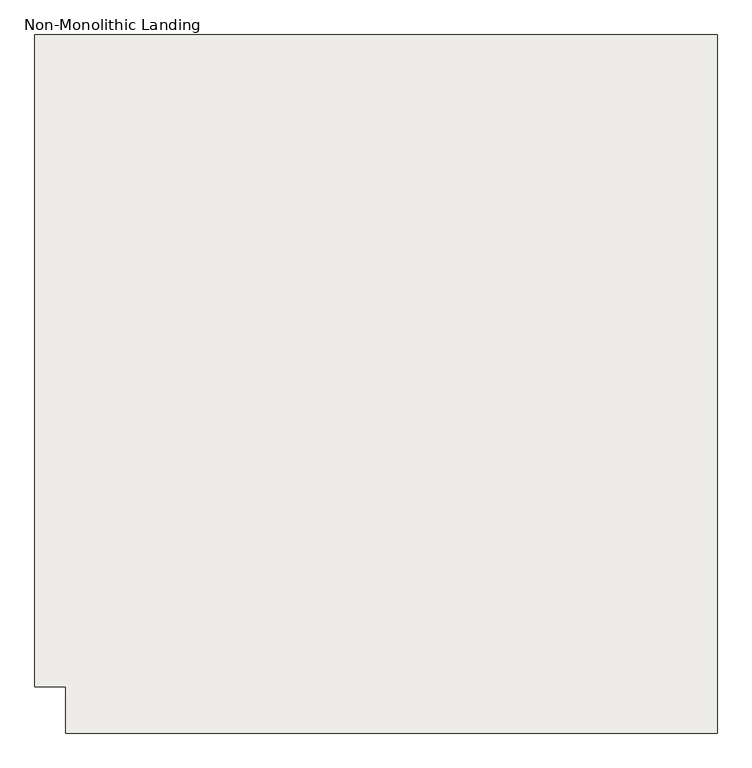
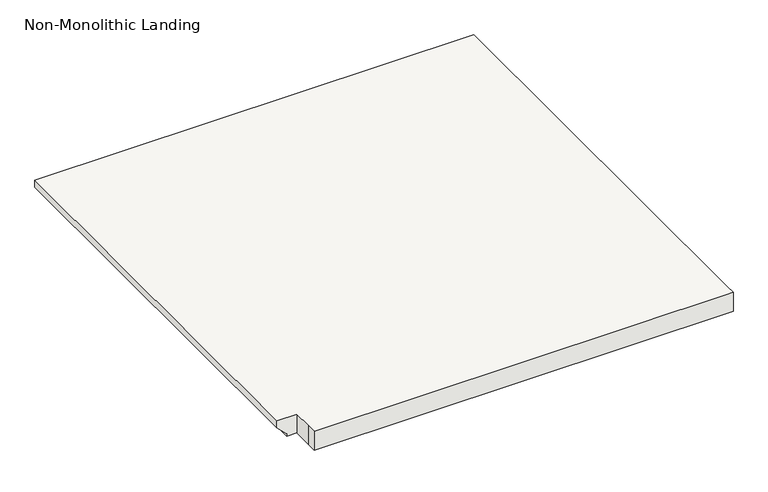
"""IFC4 building model written with IfcOpenShell, lengths in millimetres: slab geometry, Non-Monolithic Landing."""

from ifc_helpers import new_model, si_unit, origin, place, context, project, spatial, faceted_brep, source, transform, mapped, element, save


def non_monolithic_landing_ee32a08e(model_context):
    return source(origin(), model_context, "Body", "Brep", [
        faceted_brep([(2334.73354, -1849.1834702, 7753.35), (2334.73354, -1849.1834702, 7772.4), (2334.73354, -782.3834702, 7772.4), (2334.73354, -782.3834702, 7753.35), (2360.13354, -1849.1834702, 7727.95), (2360.13354, -782.3834702, 7727.95), (2385.53354, -1849.1834702, 7772.4), (2385.53354, -1899.9834702, 7772.4), (2385.53354, -1925.3834702, 7772.4), (3452.33354, -1925.3834702, 7772.4), (3452.33354, -1899.9834702, 7772.4), (3452.33354, -782.3834702, 7772.4), (2360.13354, -1849.1834702, 7721.6), (2360.13354, -782.3834702, 7721.6), (3452.33354, -782.3834702, 7721.6), (3452.33354, -1899.9834702, 7721.6), (3452.33354, -1925.3834702, 7721.6), (2385.53354, -1925.3834702, 7721.6), (2385.53354, -1899.9834702, 7721.6), (2385.53354, -1849.1834702, 7721.6)], [[[0, 1, 2, 3]], [[4, 0, 3, 5]], [[6, 7, 8, 9, 10, 11, 2, 1]], [[12, 13, 14, 15, 16, 17, 18, 19]], [[13, 12, 4, 5]], [[6, 1, 0, 4, 12, 19]], [[7, 6, 19, 18]], [[8, 7, 18, 17]], [[9, 8, 17, 16]], [[10, 9, 16, 15]], [[11, 10, 15, 14]], [[2, 11, 14, 13, 5, 3]]]),
    ])


if __name__ == "__main__":
    model = new_model("IFC4")
    model_context = context("Model", 3, world=origin())
    ifc_project = project(units=[si_unit("LENGTHUNIT", "METRE", prefix="MILLI")], contexts=[model_context])
    site = spatial("IfcSite", under=ifc_project)
    building = spatial("IfcBuilding", under=site)
    placement = place(None, origin())
    non_monolithic_landing_shape = non_monolithic_landing_ee32a08e(model_context)
    element("IfcSlab", 1, ObjectType="Non-Monolithic Landing", at=placement, inside=building, context=model_context, shape_type="MappedRepresentation", body=[
        mapped(non_monolithic_landing_shape, transform((0.0, 0.0, 0.0), x_axis=(1.0, 0.0, 0.0), y_axis=(0.0, 1.0, 0.0), z_axis=(0.0, 0.0, 1.0))),
    ])
    save(model, "model.ifc")
